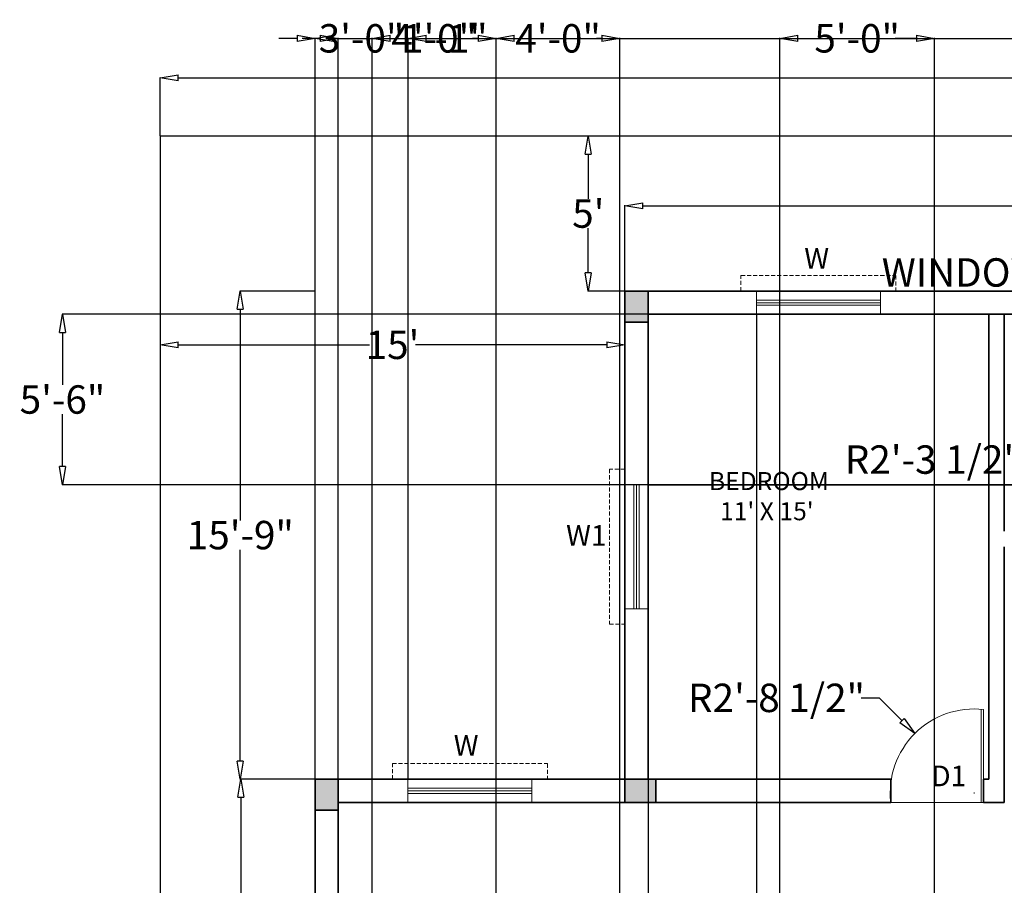
# Model space of a CAD drawing. Units: inches. Extents: x 668 to 1552, y 994 to 1684.
# Tile 2 of 4: x 680 to 1061, y 1349 to 1684. Entities that reach past the tile are written whole.
import ezdxf

# ---------------------------------------------------------------- set-up
doc = ezdxf.new("R2010")
doc.units = ezdxf.units.IN
doc.header["$LTSCALE"] = 2.5
doc.header["$MEASUREMENT"] = 0
doc.linetypes.add('HIDDEN', pattern=[0.375, 0.25, -0.125])
for name, color, linetype, lineweight, true_color in [('A-ANNO-DIMS', 175, 'Continuous', 13, 0x4554a5), ('A-ANNO-TEXT', 52, 'Continuous', 18, 0xc8c92d), ('A-DOOR', 152, 'Continuous', 18, 0x2776bb)]:
    doc.layers.add(name, color=color, linetype=linetype, lineweight=lineweight, true_color=true_color)
for name, color, linetype, lineweight in [('A-AREA-IDEN', 2, 'Continuous', 18), ('A-COLS', 7, 'Continuous', 35), ('A-COLS-PATT', 1, 'Continuous', 13), ('A-GLAZ', 4, 'Continuous', 18), ('A-WALL', 7, 'Continuous', 35), ('C-PROP', 1, 'Continuous', 25), ('sajjas', 210, 'HIDDEN', 13)]:
    doc.layers.add(name, color=color, linetype=linetype, lineweight=lineweight)
doc.styles.get("Standard").update_dxf_attribs({"font": 'arial.ttf'})
doc.dimstyles.get("Standard").update_dxf_attribs({"dimtxt": 11, "dimasz": 7, "dimexe": 0.18, "dimexo": 0.0625, "dimgap": 0.09, "dimtad": 0, "dimtih": 1, "dimtoh": 1, "dimdec": 0, "dimzin": 0, "dimdsep": 46, "dimlunit": 3, "dimtxsty": 'Standard', "dimblk": 'CLOSEDBLANK', "dimcen": 0.09, "dimadec": 0, "dimazin": 0, "dimtfac": 1, "dimtdec": 0, "dimtofl": 0, "dimtmove": 0, "dimatfit": 3, "dimldrblk": 'CLOSEDBLANK', "dimfxl": 1, "dimtolj": 1, "dimtzin": 0, "dimarcsym": 0})

# ---------------------------------------------------------------- blocks, each defined once
blk = doc.blocks.new('_ClosedBlank')
at = {"color": 0, "linetype": 'ByBlock', "lineweight": -2}
for p, q in [((-1, 0.167), (0, 0)), ((-1, 0.167), (-1, -0.167)), ((0, 0), (-1, -0.167))]:
    blk.add_line(p, q, dxfattribs=at)
blk = doc.blocks.new('*D1')
at = {"layer": 'A-ANNO-DIMS', "color": 0, "lineweight": -2, "ltscale": 2.5, "transparency": 16777216}
for p, q in [((734.36, 1639.41), (734.36, 1662.1)), ((741.36, 1661.92), (1084.91, 1661.92)), ((1447.36, 1661.92), (1103.82, 1661.92)), ((1454.36, 1639.41), (1454.36, 1662.1))]:
    blk.add_line(p, q, dxfattribs=at)
at = {"layer": 'Defpoints', "color": 0, "ltscale": 2.5, "transparency": 16777216}
for p in [(1454.36, 1661.92), (734.36, 1639.35), (1454.36, 1639.35)]:
    blk.add_point(p, dxfattribs=at)
at = {"layer": 'A-ANNO-DIMS', "color": 0, "lineweight": -2, "ltscale": 2.5, "transparency": 16777216, "xscale": 7, "yscale": 7, "zscale": 7, "rotation": 180}
blk.add_blockref('_ClosedBlank', (734.36, 1661.92), dxfattribs=at)
at = {"layer": 'A-ANNO-DIMS', "color": 0, "lineweight": -2, "ltscale": 2.5, "transparency": 16777216, "xscale": 7, "yscale": 7, "zscale": 7}
blk.add_blockref('_ClosedBlank', (1454.36, 1661.92), dxfattribs=at)
at = {"layer": 'A-ANNO-DIMS', "color": 0, "ltscale": 2.5, "transparency": 16777216, "insert": (1094.36, 1661.92), "char_height": 11, "attachment_point": 5}
blk.add_mtext("\\A1;60'", dxfattribs=at)
blk = doc.blocks.new('*D3')
at = {"layer": 'A-ANNO-DIMS', "color": 0, "lineweight": -2, "ltscale": 2.5, "transparency": 16777216}
for p, q in [((914.36, 1579.41), (914.36, 1612.58)), ((921.36, 1612.4), (1144.72, 1612.4)), ((1387.36, 1612.4), (1164.01, 1612.4)), ((1394.36, 1579.41), (1394.36, 1612.58))]:
    blk.add_line(p, q, dxfattribs=at)
at = {"layer": 'Defpoints', "color": 0, "ltscale": 2.5, "transparency": 16777216}
for p in [(914.36, 1612.4), (914.36, 1579.35), (1394.36, 1579.35)]:
    blk.add_point(p, dxfattribs=at)
at = {"layer": 'A-ANNO-DIMS', "color": 0, "lineweight": -2, "ltscale": 2.5, "transparency": 16777216, "xscale": 7, "yscale": 7, "zscale": 7, "rotation": 180}
blk.add_blockref('_ClosedBlank', (914.36, 1612.4), dxfattribs=at)
at = {"layer": 'A-ANNO-DIMS', "color": 0, "lineweight": -2, "ltscale": 2.5, "transparency": 16777216, "xscale": 7, "yscale": 7, "zscale": 7}
blk.add_blockref('_ClosedBlank', (1394.36, 1612.4), dxfattribs=at)
at = {"layer": 'A-ANNO-DIMS', "color": 0, "ltscale": 2.5, "transparency": 16777216, "insert": (1154.36, 1612.4), "char_height": 11, "attachment_point": 5}
blk.add_mtext("\\A1;40'", dxfattribs=at)
blk = doc.blocks.new('*D4')
at = {"layer": 'A-ANNO-DIMS', "color": 0, "lineweight": -2, "ltscale": 2.5, "transparency": 16777216}
for p, q in [((734.36, 1567.29), (734.36, 1558.35)), ((914.36, 1567.29), (914.36, 1558.35)), ((741.36, 1558.53), (815.46, 1558.53)), ((907.36, 1558.53), (833.27, 1558.53))]:
    blk.add_line(p, q, dxfattribs=at)
at = {"layer": 'Defpoints', "color": 0, "ltscale": 2.5, "transparency": 16777216}
for p in [(734.36, 1567.35), (914.36, 1567.35), (734.36, 1558.53)]:
    blk.add_point(p, dxfattribs=at)
at = {"layer": 'A-ANNO-DIMS', "color": 0, "lineweight": -2, "ltscale": 2.5, "transparency": 16777216, "xscale": 7, "yscale": 7, "zscale": 7, "rotation": 180}
blk.add_blockref('_ClosedBlank', (734.36, 1558.53), dxfattribs=at)
at = {"layer": 'A-ANNO-DIMS', "color": 0, "lineweight": -2, "ltscale": 2.5, "transparency": 16777216, "xscale": 7, "yscale": 7, "zscale": 7}
blk.add_blockref('_ClosedBlank', (914.36, 1558.53), dxfattribs=at)
at = {"layer": 'A-ANNO-DIMS', "color": 0, "ltscale": 2.5, "transparency": 16777216, "insert": (824.36, 1558.53), "char_height": 11, "attachment_point": 5}
blk.add_mtext("\\A1;15'", dxfattribs=at)
blk = doc.blocks.new('*D5')
at = {"layer": 'A-ANNO-DIMS', "color": 0, "lineweight": -2, "ltscale": 2.5, "transparency": 16777216}
for p, q in [((794.3, 1390.35), (765.38, 1390.35)), ((765.56, 1383.35), (765.56, 1280.56)), ((765.56, 1166.35), (765.56, 1269.14)), ((794.3, 1159.35), (765.38, 1159.35))]:
    blk.add_line(p, q, dxfattribs=at)
at = {"layer": 'Defpoints', "color": 0, "ltscale": 2.5, "transparency": 16777216}
for p in [(765.56, 1390.35), (794.36, 1390.35), (794.36, 1159.35)]:
    blk.add_point(p, dxfattribs=at)
at = {"layer": 'A-ANNO-DIMS', "color": 0, "lineweight": -2, "ltscale": 2.5, "transparency": 16777216, "xscale": 7, "yscale": 7, "zscale": 7}
for p, rotation in [((765.56, 1390.35), 90), ((765.56, 1159.35), 270)]:
    blk.add_blockref('_ClosedBlank', p, dxfattribs=dict(at, rotation=rotation))
at = {"layer": 'A-ANNO-DIMS', "color": 0, "ltscale": 2.5, "transparency": 16777216, "insert": (765.56, 1274.85), "char_height": 11, "attachment_point": 5}
blk.add_mtext('\\A1;19\'-3"', dxfattribs=at)
blk = doc.blocks.new('*D6')
at = {"layer": 'A-ANNO-DIMS', "color": 0, "lineweight": -2, "ltscale": 2.5, "transparency": 16777216}
for p, q in [((794.3, 1579.35), (765.2, 1579.35)), ((765.38, 1572.35), (765.38, 1490.56)), ((765.38, 1397.35), (765.38, 1479.14)), ((794.3, 1390.35), (765.2, 1390.35))]:
    blk.add_line(p, q, dxfattribs=at)
at = {"layer": 'Defpoints', "color": 0, "ltscale": 2.5, "transparency": 16777216}
for p in [(765.38, 1579.35), (794.36, 1579.35), (794.36, 1390.35)]:
    blk.add_point(p, dxfattribs=at)
at = {"layer": 'A-ANNO-DIMS', "color": 0, "lineweight": -2, "ltscale": 2.5, "transparency": 16777216, "xscale": 7, "yscale": 7, "zscale": 7}
for p, rotation in [((765.38, 1579.35), 90), ((765.38, 1390.35), 270)]:
    blk.add_blockref('_ClosedBlank', p, dxfattribs=dict(at, rotation=rotation))
at = {"layer": 'A-ANNO-DIMS', "color": 0, "ltscale": 2.5, "transparency": 16777216, "insert": (765.38, 1484.85), "char_height": 11, "attachment_point": 5}
blk.add_mtext('\\A1;15\'-9"', dxfattribs=at)
blk = doc.blocks.new('*D7')
at = {"layer": 'A-ANNO-DIMS', "color": 0, "lineweight": -2, "ltscale": 2.5, "transparency": 16777216}
for p, q in [((914.3, 1639.35), (900.03, 1639.35)), ((900.21, 1632.35), (900.21, 1615.03)), ((900.21, 1586.35), (900.21, 1603.67)), ((914.3, 1579.35), (900.03, 1579.35))]:
    blk.add_line(p, q, dxfattribs=at)
at = {"layer": 'Defpoints', "color": 0, "ltscale": 2.5, "transparency": 16777216}
for p in [(900.21, 1639.35), (914.36, 1639.35), (914.36, 1579.35)]:
    blk.add_point(p, dxfattribs=at)
at = {"layer": 'A-ANNO-DIMS', "color": 0, "lineweight": -2, "ltscale": 2.5, "transparency": 16777216, "xscale": 7, "yscale": 7, "zscale": 7}
for p, rotation in [((900.21, 1639.35), 90), ((900.21, 1579.35), 270)]:
    blk.add_blockref('_ClosedBlank', p, dxfattribs=dict(at, rotation=rotation))
at = {"layer": 'A-ANNO-DIMS', "color": 0, "ltscale": 2.5, "transparency": 16777216, "insert": (900.21, 1609.35), "char_height": 11, "attachment_point": 5}
blk.add_mtext("\\A1;5'", dxfattribs=at)
blk = doc.blocks.new('WIN-48')
for p, q in [((0, 9), (48, 9)), ((0, 9), (0, 0)), ((48, 9), (48, 0)), ((48, 5.5), (0, 5.5)), ((48, 4.5), (0, 4.5)), ((48, 3.5), (0, 3.5)), ((0, 0), (48, 0))]:
    blk.add_line(p, q)
blk = doc.blocks.new('SAJJA-60')
at = {"ltscale": 2.5}
blk.add_lwpolyline([(6, 6), (0, 6), (0, 0), (54, 0), (60, 0), (60, 6), (54, 6)], dxfattribs=at)
blk = doc.blocks.new('*D22')
at = {"layer": 'A-ANNO-DIMS', "color": 0, "lineweight": -2, "ltscale": 2.5, "transparency": 16777216}
for p, q in [((1157.36, 1579.41), (1157.36, 1586.73)), ((1205.36, 1579.41), (1205.36, 1586.73)), ((1157.36, 1586.55), (1150.36, 1586.55)), ((1198.36, 1586.55), (1164.36, 1586.55))]:
    blk.add_line(p, q, dxfattribs=at)
at = {"layer": 'Defpoints', "color": 0, "ltscale": 2.5, "transparency": 16777216}
for p in [(1157.36, 1586.55), (1157.36, 1579.35), (1205.36, 1579.35)]:
    blk.add_point(p, dxfattribs=at)
at = {"layer": 'A-ANNO-DIMS', "color": 0, "lineweight": -2, "ltscale": 2.5, "transparency": 16777216, "xscale": 7, "yscale": 7, "zscale": 7, "rotation": 180}
blk.add_blockref('_ClosedBlank', (1157.36, 1586.55), dxfattribs=at)
at = {"layer": 'A-ANNO-DIMS', "color": 0, "lineweight": -2, "ltscale": 2.5, "transparency": 16777216, "xscale": 7, "yscale": 7, "zscale": 7}
blk.add_blockref('_ClosedBlank', (1205.36, 1586.55), dxfattribs=at)
at = {"layer": 'A-ANNO-DIMS', "color": 0, "ltscale": 2.5, "transparency": 16777216, "insert": (1080.67, 1586.55), "char_height": 11, "attachment_point": 5}
blk.add_mtext('\\A1;WINDOW 4\'-0" TYP.', dxfattribs=at)
blk = doc.blocks.new('*D34')
at = {"layer": 'A-ANNO-DIMS', "color": 0, "lineweight": -2, "ltscale": 2.5, "transparency": 16777216}
for p, q in [((794.36, 1390.41), (794.36, 1677.38)), ((801.36, 1677.2), (1075.38, 1677.2)), ((1387.36, 1677.2), (1113.35, 1677.2)), ((1394.36, 1579.41), (1394.36, 1677.38))]:
    blk.add_line(p, q, dxfattribs=at)
at = {"layer": 'Defpoints', "color": 0, "ltscale": 2.5, "transparency": 16777216}
for p in [(1394.36, 1677.2), (1394.36, 1579.35), (794.36, 1390.35)]:
    blk.add_point(p, dxfattribs=at)
at = {"layer": 'A-ANNO-DIMS', "color": 0, "lineweight": -2, "ltscale": 2.5, "transparency": 16777216, "xscale": 7, "yscale": 7, "zscale": 7, "rotation": 180}
blk.add_blockref('_ClosedBlank', (794.36, 1677.2), dxfattribs=at)
at = {"layer": 'A-ANNO-DIMS', "color": 0, "lineweight": -2, "ltscale": 2.5, "transparency": 16777216, "xscale": 7, "yscale": 7, "zscale": 7}
blk.add_blockref('_ClosedBlank', (1394.36, 1677.2), dxfattribs=at)
at = {"layer": 'A-ANNO-DIMS', "color": 0, "ltscale": 2.5, "transparency": 16777216, "insert": (1094.36, 1677.2), "char_height": 11, "attachment_point": 5}
blk.add_mtext('\\A1;50\'-0"', dxfattribs=at)
blk = doc.blocks.new('*D37')
at = {"layer": 'A-ANNO-DIMS', "color": 0, "lineweight": -2, "ltscale": 2.5, "transparency": 16777216}
for p, q in [((974.36, 1168.41), (974.36, 1677.38)), ((981.36, 1677.2), (989.65, 1677.2)), ((1027.36, 1677.2), (1019.07, 1677.2)), ((1034.36, 1168.41), (1034.36, 1677.38))]:
    blk.add_line(p, q, dxfattribs=at)
at = {"layer": 'Defpoints', "color": 0, "ltscale": 2.5, "transparency": 16777216}
for p in [(1034.36, 1677.2), (974.36, 1168.35), (1034.36, 1168.35)]:
    blk.add_point(p, dxfattribs=at)
at = {"layer": 'A-ANNO-DIMS', "color": 0, "lineweight": -2, "ltscale": 2.5, "transparency": 16777216, "xscale": 7, "yscale": 7, "zscale": 7, "rotation": 180}
blk.add_blockref('_ClosedBlank', (974.36, 1677.2), dxfattribs=at)
at = {"layer": 'A-ANNO-DIMS', "color": 0, "lineweight": -2, "ltscale": 2.5, "transparency": 16777216, "xscale": 7, "yscale": 7, "zscale": 7}
blk.add_blockref('_ClosedBlank', (1034.36, 1677.2), dxfattribs=at)
at = {"layer": 'A-ANNO-DIMS', "color": 0, "ltscale": 2.5, "transparency": 16777216, "insert": (1004.36, 1677.2), "char_height": 11, "attachment_point": 5}
blk.add_mtext('\\A1;5\'-0"', dxfattribs=at)
blk = doc.blocks.new('*D38')
at = {"layer": 'A-ANNO-DIMS', "color": 0, "lineweight": -2, "ltscale": 2.5, "transparency": 16777216}
for p, q in [((923.362549, 1570.287512), (923.362549, 1001.320012)), ((965.362549, 1570.287512), (965.362549, 1001.320012)), ((916.362549, 1001.500012), (909.362549, 1001.500012)), ((972.362549, 1001.500012), (979.362549, 1001.500012))]:
    blk.add_line(p, q, dxfattribs=at)
at = {"layer": 'Defpoints', "color": 0, "ltscale": 2.5, "transparency": 16777216}
for p in [(923.362549, 1570.350012), (965.362549, 1570.350012), (965.362549, 1001.500012)]:
    blk.add_point(p, dxfattribs=at)
at = {"layer": 'A-ANNO-DIMS', "color": 0, "lineweight": -2, "ltscale": 2.5, "transparency": 16777216, "xscale": 7, "yscale": 7, "zscale": 7}
blk.add_blockref('_ClosedBlank', (923.362549, 1001.500012), dxfattribs=at)
at = {"layer": 'A-ANNO-DIMS', "color": 0, "lineweight": -2, "ltscale": 2.5, "transparency": 16777216, "xscale": 7, "yscale": 7, "zscale": 7, "rotation": 180}
blk.add_blockref('_ClosedBlank', (965.362549, 1001.500012), dxfattribs=at)
at = {"layer": 'A-ANNO-DIMS', "color": 0, "ltscale": 2.5, "transparency": 16777216, "insert": (944.362549, 1001.500012), "char_height": 11, "attachment_point": 5}
blk.add_mtext('\\A1;3\'-6"', dxfattribs=at)
blk = doc.blocks.new('*D42')
at = {"layer": 'A-ANNO-DIMS', "color": 0, "lineweight": -2, "ltscale": 2.5, "transparency": 16777216}
for p, q in [((1385.3, 1570.35), (696.33, 1570.35)), ((696.51, 1563.35), (696.51, 1543.06)), ((696.51, 1511.35), (696.51, 1531.64)), ((1385.3, 1504.35), (696.33, 1504.35))]:
    blk.add_line(p, q, dxfattribs=at)
at = {"layer": 'Defpoints', "color": 0, "ltscale": 2.5, "transparency": 16777216}
for p in [(1385.36, 1570.35), (696.51, 1504.35), (1385.36, 1504.35)]:
    blk.add_point(p, dxfattribs=at)
at = {"layer": 'A-ANNO-DIMS', "color": 0, "lineweight": -2, "ltscale": 2.5, "transparency": 16777216, "xscale": 7, "yscale": 7, "zscale": 7}
for p, rotation in [((696.51, 1570.35), 90), ((696.51, 1504.35), 270)]:
    blk.add_blockref('_ClosedBlank', p, dxfattribs=dict(at, rotation=rotation))
at = {"layer": 'A-ANNO-DIMS', "color": 0, "ltscale": 2.5, "transparency": 16777216, "insert": (696.51, 1537.35), "char_height": 11, "attachment_point": 5}
blk.add_mtext('\\A1;5\'-6"', dxfattribs=at)
blk = doc.blocks.new('*D43')
at = {"layer": 'A-ANNO-DIMS', "color": 0, "lineweight": -2, "ltscale": 2.5, "transparency": 16777216}
for p, q in [((923.43, 1570.35), (1492.39, 1570.35)), ((1492.21, 1563.35), (1492.21, 1543.06)), ((1492.21, 1511.35), (1492.21, 1531.64)), ((923.43, 1504.35), (1492.39, 1504.35))]:
    blk.add_line(p, q, dxfattribs=at)
at = {"layer": 'Defpoints', "color": 0, "ltscale": 2.5, "transparency": 16777216}
for p in [(923.36, 1570.35), (923.36, 1504.35), (1492.21, 1504.35)]:
    blk.add_point(p, dxfattribs=at)
at = {"layer": 'A-ANNO-DIMS', "color": 0, "lineweight": -2, "ltscale": 2.5, "transparency": 16777216, "xscale": 7, "yscale": 7, "zscale": 7}
for p, rotation in [((1492.21, 1570.35), 90), ((1492.21, 1504.35), 270)]:
    blk.add_blockref('_ClosedBlank', p, dxfattribs=dict(at, rotation=rotation))
at = {"layer": 'A-ANNO-DIMS', "color": 0, "ltscale": 2.5, "transparency": 16777216, "insert": (1492.21, 1537.35), "char_height": 11, "attachment_point": 5}
blk.add_mtext('\\A1;5\'-6"', dxfattribs=at)
blk = doc.blocks.new('*D44')
at = {"layer": 'A-ANNO-DIMS', "color": 0, "lineweight": -2, "ltscale": 2.5, "transparency": 16777216}
for p, q in [((787.362549, 1677.200012), (780.362549, 1677.200012)), ((794.362549, 1390.412512), (794.362549, 1677.380012)), ((830.362549, 1390.412512), (830.362549, 1677.380012)), ((837.362549, 1677.200012), (844.362549, 1677.200012))]:
    blk.add_line(p, q, dxfattribs=at)
at = {"layer": 'Defpoints', "color": 0, "ltscale": 2.5, "transparency": 16777216}
for p in [(830.362549, 1677.200012), (794.362549, 1390.350012), (830.362549, 1390.350012)]:
    blk.add_point(p, dxfattribs=at)
at = {"layer": 'A-ANNO-DIMS', "color": 0, "lineweight": -2, "ltscale": 2.5, "transparency": 16777216, "xscale": 7, "yscale": 7, "zscale": 7}
blk.add_blockref('_ClosedBlank', (794.362549, 1677.200012), dxfattribs=at)
at = {"layer": 'A-ANNO-DIMS', "color": 0, "lineweight": -2, "ltscale": 2.5, "transparency": 16777216, "xscale": 7, "yscale": 7, "zscale": 7, "rotation": 180}
blk.add_blockref('_ClosedBlank', (830.362549, 1677.200012), dxfattribs=at)
at = {"layer": 'A-ANNO-DIMS', "color": 0, "ltscale": 2.5, "transparency": 16777216, "insert": (812.362549, 1677.200012), "char_height": 11, "attachment_point": 5}
blk.add_mtext('\\A1;3\'-0"', dxfattribs=at)
blk = doc.blocks.new('*D46')
at = {"layer": 'A-ANNO-DIMS', "color": 0, "lineweight": -2, "ltscale": 2.5, "transparency": 16777216}
for p, q in [((796.36, 1677.2), (789.36, 1677.2)), ((803.36, 1168.41), (803.36, 1677.38)), ((816.48, 1168.41), (816.48, 1677.38)), ((823.48, 1677.2), (830.48, 1677.2))]:
    blk.add_line(p, q, dxfattribs=at)
at = {"layer": 'Defpoints', "color": 0, "ltscale": 2.5, "transparency": 16777216}
for p in [(816.48, 1677.2), (803.36, 1168.35), (816.48, 1168.35)]:
    blk.add_point(p, dxfattribs=at)
at = {"layer": 'A-ANNO-DIMS', "color": 0, "lineweight": -2, "ltscale": 2.5, "transparency": 16777216, "xscale": 7, "yscale": 7, "zscale": 7}
blk.add_blockref('_ClosedBlank', (803.36, 1677.2), dxfattribs=at)
at = {"layer": 'A-ANNO-DIMS', "color": 0, "lineweight": -2, "ltscale": 2.5, "transparency": 16777216, "xscale": 7, "yscale": 7, "zscale": 7, "rotation": 180}
blk.add_blockref('_ClosedBlank', (816.48, 1677.2), dxfattribs=at)
at = {"layer": 'A-ANNO-DIMS', "color": 0, "ltscale": 2.5, "transparency": 16777216, "insert": (844.67, 1677.2), "char_height": 11, "attachment_point": 5}
blk.add_mtext('\\A1;1\'-1"', dxfattribs=at)
blk = doc.blocks.new('*D47')
at = {"layer": 'A-ANNO-DIMS', "color": 0, "lineweight": -2, "ltscale": 2.5, "transparency": 16777216}
for p, q in [((816.48, 1168.41), (816.48, 1677.38)), ((823.48, 1677.2), (825.55, 1677.2)), ((857.48, 1677.2), (855.41, 1677.2)), ((864.48, 1168.41), (864.48, 1677.38))]:
    blk.add_line(p, q, dxfattribs=at)
at = {"layer": 'Defpoints', "color": 0, "ltscale": 2.5, "transparency": 16777216}
for p in [(864.48, 1677.2), (816.48, 1168.35), (864.48, 1168.35)]:
    blk.add_point(p, dxfattribs=at)
at = {"layer": 'A-ANNO-DIMS', "color": 0, "lineweight": -2, "ltscale": 2.5, "transparency": 16777216, "xscale": 7, "yscale": 7, "zscale": 7, "rotation": 180}
blk.add_blockref('_ClosedBlank', (816.48, 1677.2), dxfattribs=at)
at = {"layer": 'A-ANNO-DIMS', "color": 0, "lineweight": -2, "ltscale": 2.5, "transparency": 16777216, "xscale": 7, "yscale": 7, "zscale": 7}
blk.add_blockref('_ClosedBlank', (864.48, 1677.2), dxfattribs=at)
at = {"layer": 'A-ANNO-DIMS', "color": 0, "ltscale": 2.5, "transparency": 16777216, "insert": (840.48, 1677.2), "char_height": 11, "attachment_point": 5}
blk.add_mtext('\\A1;4\'-0"', dxfattribs=at)
blk = doc.blocks.new('*D48')
at = {"layer": 'A-ANNO-DIMS', "color": 0, "lineweight": -2, "ltscale": 2.5, "transparency": 16777216}
for p, q in [((864.48, 1168.41), (864.48, 1677.38)), ((871.48, 1677.2), (873.55, 1677.2)), ((905.48, 1677.2), (903.41, 1677.2)), ((912.48, 1168.41), (912.48, 1677.38))]:
    blk.add_line(p, q, dxfattribs=at)
at = {"layer": 'Defpoints', "color": 0, "ltscale": 2.5, "transparency": 16777216}
for p in [(912.48, 1677.2), (864.48, 1168.35), (912.48, 1168.35)]:
    blk.add_point(p, dxfattribs=at)
at = {"layer": 'A-ANNO-DIMS', "color": 0, "lineweight": -2, "ltscale": 2.5, "transparency": 16777216, "xscale": 7, "yscale": 7, "zscale": 7, "rotation": 180}
blk.add_blockref('_ClosedBlank', (864.48, 1677.2), dxfattribs=at)
at = {"layer": 'A-ANNO-DIMS', "color": 0, "lineweight": -2, "ltscale": 2.5, "transparency": 16777216, "xscale": 7, "yscale": 7, "zscale": 7}
blk.add_blockref('_ClosedBlank', (912.48, 1677.2), dxfattribs=at)
at = {"layer": 'A-ANNO-DIMS', "color": 0, "ltscale": 2.5, "transparency": 16777216, "insert": (888.48, 1677.2), "char_height": 11, "attachment_point": 5}
blk.add_mtext('\\A1;4\'-0"', dxfattribs=at)
blk = doc.blocks.new('*D56')
at = {"layer": 'A-ANNO-DIMS', "color": 0, "lineweight": -2, "ltscale": 2.5, "transparency": 16777216}
for p, q in [((1005.88, 1421.83), (1012.88, 1421.83)), ((1012.88, 1421.83), (1021.74, 1412.97)), ((1049.63, 1385), (1049.81, 1385)), ((1049.72, 1384.91), (1049.72, 1385.09))]:
    blk.add_line(p, q, dxfattribs=at)
at = {"layer": 'Defpoints', "color": 0, "ltscale": 2.5, "transparency": 16777216}
for p in [(1026.69, 1408.02), (1049.72, 1385)]:
    blk.add_point(p, dxfattribs=at)
at = {"layer": 'A-ANNO-DIMS', "color": 0, "lineweight": -2, "ltscale": 2.5, "transparency": 16777216, "xscale": 7, "yscale": 7, "zscale": 7, "rotation": 315.0006968126921}
blk.add_blockref('_ClosedBlank', (1026.69, 1408.02), dxfattribs=at)
at = {"layer": 'A-ANNO-DIMS', "color": 0, "ltscale": 2.5, "transparency": 16777216, "insert": (973.09, 1421.83), "char_height": 11, "attachment_point": 5}
blk.add_mtext('\\A1;R2\'-8 1/2"', dxfattribs=at)
blk = doc.blocks.new('*D59')
at = {"layer": 'A-ANNO-DIMS', "color": 0, "lineweight": -2, "ltscale": 2.5, "transparency": 16777216}
for p, q in [((1066.62, 1514.09), (1073.62, 1514.09)), ((1073.62, 1514.09), (1080.43, 1507.28)), ((1104.9, 1482.72), (1105.08, 1482.72)), ((1104.99, 1482.63), (1104.99, 1482.81))]:
    blk.add_line(p, q, dxfattribs=at)
at = {"layer": 'Defpoints', "color": 0, "ltscale": 2.5, "transparency": 16777216}
for p in [(1085.38, 1502.33), (1104.99, 1482.72)]:
    blk.add_point(p, dxfattribs=at)
at = {"layer": 'A-ANNO-DIMS', "color": 0, "lineweight": -2, "ltscale": 2.5, "transparency": 16777216, "xscale": 7, "yscale": 7, "zscale": 7, "rotation": 315.0008195408938}
blk.add_blockref('_ClosedBlank', (1085.38, 1502.33), dxfattribs=at)
at = {"layer": 'A-ANNO-DIMS', "color": 0, "ltscale": 2.5, "transparency": 16777216, "insert": (1033.83, 1514.09), "char_height": 11, "attachment_point": 5}
blk.add_mtext('\\A1;R2\'-3 1/2"', dxfattribs=at)

msp = doc.modelspace()

# ---------------------------------------------------------------- hatches: boundary and pattern name
at = {"layer": 'A-COLS-PATT'}
h = msp.add_hatch(color=256, dxfattribs=at)
h.dxf.hatch_style = 1
h.paths.add_polyline_path([(803.36, 1390.35), (794.36, 1390.35), (794.36, 1378.35), (803.36, 1378.35)])
h.paths.add_polyline_path([(1117.36, 1393.35), (1108.36, 1393.35), (1108.36, 1381.35), (1117.36, 1381.35)])
h.paths.add_polyline_path([(1255.36, 1390.35), (1243.36, 1390.35), (1243.36, 1381.35), (1255.36, 1381.35)])
h.paths.add_polyline_path([(1394.36, 1390.35), (1382.36, 1390.35), (1382.36, 1381.35), (1394.36, 1381.35)])
h.paths.add_polyline_path([(1394.36, 1579.35), (1385.36, 1579.35), (1385.36, 1567.35), (1394.36, 1567.35)])
h.paths.add_polyline_path([(1253.36, 1579.35), (1241.36, 1579.35), (1241.36, 1570.35), (1253.36, 1570.35)])
h.paths.add_polyline_path([(1115.36, 1579.35), (1103.36, 1579.35), (1103.36, 1570.35), (1115.36, 1570.35)])
h.paths.add_polyline_path([(923.36, 1579.35), (914.36, 1579.35), (914.36, 1567.35), (923.36, 1567.35)])
h.paths.add_polyline_path([(926.36, 1390.35), (914.36, 1390.35), (914.36, 1381.35), (926.36, 1381.35)])
h.paths.add_polyline_path([(1394.36, 1243.35), (1382.36, 1243.35), (1382.36, 1234.35), (1394.36, 1234.35)])
h.paths.add_polyline_path([(1277.36, 1342.35), (1265.36, 1342.35), (1265.36, 1333.35), (1277.36, 1333.35)])
h.paths.add_polyline_path([(1130.36, 1311.02), (1121.36, 1311.02), (1121.36, 1299.02), (1130.36, 1299.02)])
h.paths.add_polyline_path([(1043.36, 1311.02), (1034.36, 1311.02), (1034.36, 1299.02), (1043.36, 1299.02)])
h.paths.add_polyline_path([(803.36, 1171.35), (794.36, 1171.35), (794.36, 1159.35), (803.36, 1159.35)])
h.paths.add_polyline_path([(1046.36, 1168.35), (1034.36, 1168.35), (1034.36, 1159.35), (1046.36, 1159.35)])
h.paths.add_polyline_path([(1133.36, 1168.35), (1121.36, 1168.35), (1121.36, 1159.35), (1133.36, 1159.35)])
h.paths.add_polyline_path([(1277.36, 1168.35), (1265.36, 1168.35), (1265.36, 1159.35), (1277.36, 1159.35)])

# ---------------------------------------------------------------- linework, layer by layer
at = {"layer": 'A-COLS'}
for points in [[(914.36, 1567.35), (923.36, 1567.35), (923.36, 1579.35), (914.36, 1579.35)], [(794.36, 1378.35), (803.36, 1378.35), (803.36, 1390.35), (794.36, 1390.35)], [(926.36, 1381.35), (926.36, 1390.35), (914.36, 1390.35), (914.36, 1381.35)]]:
    msp.add_lwpolyline(points, close=True, dxfattribs=at)
at = {"layer": 'A-DOOR'}
for p, q in [((1052.36, 1381.35), (1052.36, 1417.35)), ((1053.36, 1381.35), (1053.36, 1417.35)), ((1017.36, 1381.35), (1053.36, 1381.35))]:
    msp.add_line(p, q, dxfattribs=at)
msp.add_arc((1049.72, 1385), 32.56, 83.5723, 186.4277, dxfattribs=at)
at = {"layer": 'A-GLAZ'}
for p, q in [((965.36, 1570.35), (965.36, 1579.35)), ((1013.36, 1570.35), (1013.36, 1579.35))]:
    msp.add_line(p, q, dxfattribs=at)
at = {"layer": 'A-WALL'}
for p, q in [((1394.36, 1579.35), (914.36, 1579.35)), ((914.36, 1390.35), (914.36, 1579.35)), ((1055.36, 1570.35), (923.36, 1570.35)), ((923.36, 1390.35), (923.36, 1570.35)), ((1055.36, 1390.35), (1055.36, 1570.35)), ((1109.36, 1570.35), (1061.36, 1570.35)), ((1061.36, 1486.35), (1061.36, 1570.35)), ((1061.36, 1381.35), (1061.36, 1480.35)), ((794.36, 1390.35), (794.36, 1159.35)), ((914.36, 1390.35), (794.36, 1390.35)), ((1017.36, 1390.35), (923.36, 1390.35)), ((1017.36, 1390.35), (1017.36, 1381.35)), ((1055.36, 1390.35), (1053.36, 1390.35)), ((1053.36, 1390.35), (1053.36, 1381.35)), ((803.36, 1381.35), (803.36, 1168.35)), ((1017.36, 1381.35), (803.36, 1381.35)), ((1061.36, 1381.35), (1053.36, 1381.35))]:
    msp.add_line(p, q, dxfattribs=at)
at = {"layer": 'C-PROP', "ltscale": 2.5}
for p, q in [((1454.36, 1639.35), (734.36, 1639.35)), ((734.36, 1639.35), (734.36, 1039.35))]:
    msp.add_line(p, q, dxfattribs=at)

# ---------------------------------------------------------------- block references
at = {"layer": 'A-GLAZ'}
for p, rotation in [((1013.36, 1579.35), 180), ((914.36, 1504.35), 270.0000000000013)]:
    msp.add_blockref('WIN-48', p, dxfattribs=dict(at, rotation=rotation))
msp.add_blockref('WIN-48', (830.36, 1381.35), dxfattribs=at)
at = {"layer": 'sajjas', "extrusion": (0, 0, -1), "zscale": -1, "rotation": 180}
for p in [(-959.36, 1585.35), (-824.36, 1396.35)]:
    msp.add_blockref('SAJJA-60', p, dxfattribs=at)
at = {"layer": 'sajjas', "rotation": 269.9999999999999}
msp.add_blockref('SAJJA-60', (908.36, 1510.35), dxfattribs=at)

# ---------------------------------------------------------------- texts
at = {"layer": 'A-ANNO-TEXT', "ltscale": 2.5, "char_height": 8, "attachment_point": 1}
for s, insert in [('W', (983.88, 1595.99)), ('W1', (891.62, 1488.7)), ('W', (848.09, 1407.41)), ('D1', (1033.06, 1395.59))]:
    msp.add_mtext_dynamic_manual_height_columns(s, width=96.0512, gutter_width=1, heights=[0], dxfattribs=dict(at, insert=insert))
at = {"layer": 'A-AREA-IDEN', "ltscale": 2.5, "insert": (946.96, 1509.27), "char_height": 7, "attachment_point": 1}
msp.add_mtext_dynamic_manual_height_columns("BEDROOM\\P  11' X 15'", width=47.3322, gutter_width=1, heights=[0], dxfattribs=at)

# ---------------------------------------------------------------- dimensions: what is measured, and where the dimension line sits
at = {"layer": 'A-ANNO-DIMS', "ltscale": 2.5}
for base, p1, p2, override, picture, middle in [((830.36, 1677.2), (794.36, 1390.35), (830.36, 1390.35), {"dimdec": 1, "dimlfac": 1, "dimrnd": 0, "dimzin": 1, "dimdsep": 46, "dimlunit": 4, "dimfrac": 2}, '*D44', (812.36, 1677.2)), ((816.48, 1677.2), (803.36, 1168.35), (816.48, 1168.35), {"dimdec": 1, "dimlfac": 1, "dimrnd": 0, "dimzin": 1, "dimdsep": 46, "dimlunit": 4, "dimfrac": 2}, '*D46', (844.67, 1677.2)), ((1394.36, 1677.2), (794.36, 1390.35), (1394.36, 1579.35), {"dimdec": 1, "dimlfac": 1, "dimrnd": 0, "dimzin": 1, "dimdsep": 46, "dimlunit": 4, "dimfrac": 2}, '*D34', (1094.36, 1677.2)), ((864.48, 1677.2), (816.48, 1168.35), (864.48, 1168.35), {"dimdec": 1, "dimlfac": 1, "dimrnd": 0, "dimzin": 1, "dimdsep": 46, "dimlunit": 4, "dimfrac": 2}, '*D47', (840.48, 1677.2)), ((912.48, 1677.2), (864.48, 1168.35), (912.48, 1168.35), {"dimdec": 1, "dimlfac": 1, "dimrnd": 0, "dimzin": 1, "dimdsep": 46, "dimlunit": 4, "dimfrac": 2}, '*D48', (888.48, 1677.2)), ((1034.36, 1677.2), (974.36, 1168.35), (1034.36, 1168.35), {"dimdec": 1, "dimlfac": 1, "dimrnd": 0, "dimzin": 1, "dimdsep": 46, "dimlunit": 4, "dimfrac": 2}, '*D37', (1004.36, 1677.2)), ((1454.36, 1661.92), (734.36, 1639.35), (1454.36, 1639.35), {"dimclrd": 0, "dimclre": 0, "dimclrt": 0}, '*D1', (1094.36, 1661.92)), ((914.36, 1612.4), (1394.36, 1579.35), (914.36, 1579.35), {"dimclrd": 0, "dimclre": 0, "dimclrt": 0}, '*D3', (1154.36, 1612.4)), ((965.36, 1001.5), (923.36, 1570.35), (965.36, 1570.35), {"dimdec": 1, "dimlfac": 1, "dimrnd": 0, "dimzin": 1, "dimdsep": 46, "dimlunit": 4, "dimfrac": 2}, '*D38', (944.36, 1001.5)), ((734.36, 1558.53), (914.36, 1567.35), (734.36, 1567.35), {"dimclrd": 0, "dimclre": 0, "dimclrt": 0}, '*D4', (824.36, 1558.53))]:
    dim = msp.add_linear_dim(base=base, p1=p1, p2=p2, dimstyle='Standard', override=override, dxfattribs=at)
    dim.commit()
    dim.dimension.update_dxf_attribs({"geometry": picture, "text_midpoint": middle})
for base, p1, p2, override, picture, middle in [((900.21, 1639.35), (914.36, 1579.35), (914.36, 1639.35), {"dimclrd": 0, "dimclre": 0, "dimclrt": 0}, '*D7', (900.21, 1609.35)), ((765.38, 1579.35), (794.36, 1390.35), (794.36, 1579.35), {"dimclrd": 0, "dimclre": 0, "dimclrt": 0}, '*D6', (765.38, 1484.85)), ((696.51, 1504.35), (1385.36, 1570.35), (1385.36, 1504.35), {"dimdec": 1, "dimlfac": 1, "dimrnd": 0, "dimzin": 1, "dimdsep": 46, "dimlunit": 4, "dimfrac": 2}, '*D42', (696.51, 1537.35)), ((1492.21, 1504.35), (923.36, 1570.35), (923.36, 1504.35), {"dimdec": 1, "dimlfac": 1, "dimrnd": 0, "dimzin": 1, "dimdsep": 46, "dimlunit": 4, "dimfrac": 2}, '*D43', (1492.21, 1537.35)), ((765.56, 1390.35), (794.36, 1159.35), (794.36, 1390.35), {"dimclrd": 0, "dimclre": 0, "dimclrt": 0}, '*D5', (765.56, 1274.85))]:
    dim = msp.add_linear_dim(base=base, p1=p1, p2=p2, angle=90, dimstyle='Standard', override=override, dxfattribs=at)
    dim.commit()
    dim.dimension.update_dxf_attribs({"geometry": picture, "text_midpoint": middle})
dim = msp.add_linear_dim(base=(1157.36, 1586.55), p1=(1205.36, 1579.35), p2=(1157.36, 1579.35), angle=180, text='WINDOW <> TYP.', dimstyle='Standard', override={"dimdec": 1, "dimlfac": 1, "dimrnd": 0, "dimzin": 1, "dimdsep": 46, "dimlunit": 4, "dimfrac": 2}, dxfattribs=at)
dim.commit()
dim.dimension.update_dxf_attribs({"geometry": '*D22', "text_midpoint": (1080.67, 1586.55)})
for center, mpoint, picture, middle in [((1104.99, 1482.72), (1085.38, 1502.33), '*D59', (1033.83, 1514.09)), ((1049.72, 1385), (1026.69, 1408.02), '*D56', (973.09, 1421.83))]:
    dim = msp.add_radius_dim(center=center, mpoint=mpoint, dimstyle='Standard', override={"dimdec": 1, "dimlfac": 1, "dimrnd": 0, "dimzin": 1, "dimdsep": 46, "dimlunit": 4, "dimfrac": 2}, dxfattribs=at)
    dim.commit()
    dim.dimension.update_dxf_attribs({"geometry": picture, "text_midpoint": middle, "dimtype": 164})

doc.saveas('drawing.dxf')
